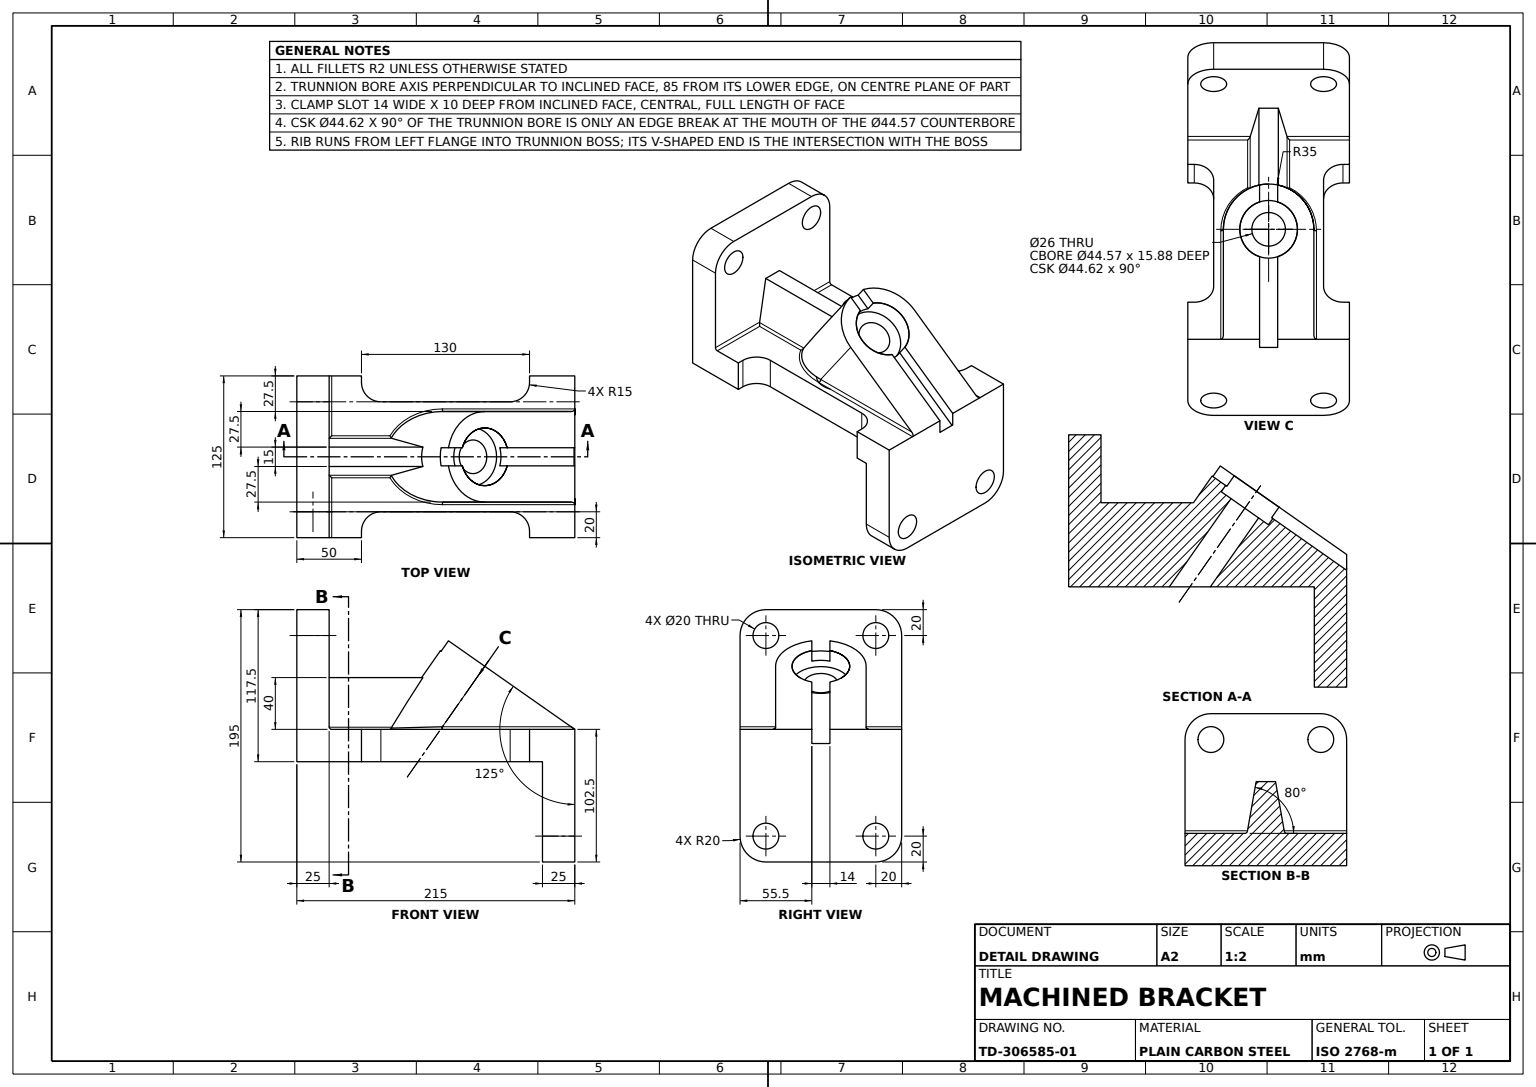
SolidWorks part; units mm, degrees
material "Plain Carbon Steel"
ref_plane "Front Plane" through (0, 0, 0) normal (0, 0, 1) x (1, 0, 0)
ref_plane "Top Plane" through (0, 0, 0) normal (0, 1, 0) x (1, 0, 0)
ref_plane "Right Plane" through (0, 0, 0) normal (1, 0, 0) x (0, 0, -1)
sketch "Base Plate Sketch" plane through (0, 0, 0) normal (0, 1, 0) x (1, 0, 0)
  line L0 (72.5, 62.5) -> (107.5, 62.5)
  line L1 (-107.5, -62.5) -> (-57.5, -62.5)
  line L2 (-107.5, -62.5) -> (-107.5, 62.5)
  line L3 (-107.5, 62.5) -> (-57.5, 62.5)
  line L4 (107.5, -62.5) -> (107.5, 62.5)
  line L5 (-107.5, -62.5) -> (107.5, 62.5) construction
  line L6 (-107.5, 62.5) -> (107.5, -62.5) construction
  line L8 (72.5, 62.5) -> (72.5, 57.5)
  line L9 (57.5, 42.5) -> (-42.5, 42.5)
  line L10 (-57.5, 62.5) -> (-57.5, 57.5)
  line L11 (0, 0) -> (-93.3615, 0) construction
  line L12 (-57.5, -62.5) -> (-57.5, -57.5)
  line L13 (72.5, -62.5) -> (72.5, -57.5)
  line L14 (57.5, -42.5) -> (-42.5, -42.5)
  line L15 (72.5, -62.5) -> (107.5, -62.5)
  arc A0 (-57.5, 57.5) -> (-42.5, 42.5) centre (-42.5, 57.5) ccw
  arc A1 (57.5, 42.5) -> (72.5, 57.5) centre (57.5, 57.5) ccw
  arc A2 (-57.5, -57.5) -> (-42.5, -42.5) centre (-42.5, -57.5) cw
  arc A3 (57.5, -42.5) -> (72.5, -57.5) centre (57.5, -57.5) cw
  point P0 (0, 0)
  point P13 (-57.5, 42.5)
  point P16 (72.5, 42.5)
  dimension "D5" = 15
  dimension "D1" = 215
  dimension "D2" = 125
  dimension "D3" = 20
  dimension "D4" = 100
  dimension "D6" = 50
extrude "Base Plate" add sketch "Base Plate Sketch" along normal blind 25
sketch "End Flange A Sketch" plane through (107.5, 0, 0) normal (1, 0, 0) x (0, 0, -1)
  line L0 (62.5, 25) -> (62.5, 0) construction
  line L1 (-62.5, 25) -> (62.5, 25)
  line L2 (-62.5, 25) -> (-62.5, -57.5)
  line L3 (-42.5, -77.5) -> (42.5, -77.5)
  line L4 (62.5, 25) -> (62.5, -57.5)
  arc A0 (62.5, -57.5) -> (42.5, -77.5) centre (42.5, -57.5) cw
  arc A1 (-42.5, -77.5) -> (-62.5, -57.5) centre (-42.5, -57.5) cw
  circle A2 centre (-42.5, -57.5) radius 10
  circle A3 centre (42.5, -57.5) radius 10
  dimension "D2" = 20
  dimension "D3" = 20
  dimension "D1" = 102.5
extrude "End Flange A" add sketch "End Flange A Sketch" against normal blind 25
sketch "End Flange B Sketch" plane through (-107.5, 0, 0) normal (-1, 0, 0) x (0, 0, 1)
  line L0 (62.5, 25) -> (62.5, 0) construction
  line L1 (-62.5, 0) -> (62.5, 0)
  line L2 (-62.5, 0) -> (-62.5, 97.5)
  line L3 (-42.5, 117.5) -> (42.5, 117.5)
  line L4 (62.5, 0) -> (62.5, 97.5)
  arc A0 (42.5, 117.5) -> (62.5, 97.5) centre (42.5, 97.5) cw
  arc A1 (-62.5, 97.5) -> (-42.5, 117.5) centre (-42.5, 97.5) cw
  circle A2 centre (-42.5, 97.5) radius 10
  circle A3 centre (42.5, 97.5) radius 10
  point P11 (-62.5, 117.5)
  dimension "D2" = 20
  dimension "D3" = 20
  dimension "D1" = 117.5
extrude "End Flange B" add sketch "End Flange B Sketch" against normal blind 25
ref_plane "Trunnion Plane 125deg" through (47.1126, 67.2837, 0) normal (-0.5736, -0.8192, 0) x (0, 0, -1)
sketch "Trunnion Boss Sketch" plane through (47.1126, 67.2837, 0) normal (-0.5736, -0.8192, 0) x (0, 0, -1)
  line L0 (-35, -11.2806) -> (-35, 73.7194)
  line L1 (-35, 73.7194) -> (35, 73.7194)
  line L2 (35, 73.7194) -> (35, -11.2806)
  line L5 (-62.5, 73.7194) -> (62.5, 73.7194) construction
  arc A0 (-35, -11.2806) -> (35, -11.2806) centre (0, -11.2806) ccw
  dimension "D1" = 70
  dimension "D2" = 85
extrude "Angled Trunnion Boss" add sketch "Trunnion Boss Sketch" along normal up to surface up to face at (8.75, 25, 0)
hole_wizard "Trunnion Bore CBORE M24" positions "3DSketch1" profile "Sketch6" counterbore size "M24" standard "ANSI Metric" end condition through all
sketch3d "3DSketch1"
  arc A0 (37.8721, 73.754, 35) -> (37.8721, 73.754, -35) centre (37.8721, 73.754, 0) ccw construction
  point P0 (37.8721, 73.754, 0)
  point P6 (17.7969, 45.0837, 0)
sketch "Sketch6" plane through (37.8721, 73.754, 0) normal (0, 0, 1) x (-0.8192, 0.5736, 0)
  line L0 (0, 0) -> (0, 207.282)
  line L1 (0, 207.282) -> (13, 207.282)
  line L3 (13, 207.282) -> (13, 15.9)
  line L4 (22.285, 15.9) -> (13, 15.9)
  line L5 (22.285, 15.9) -> (22.285, 0.025)
  line L6 (22.285, 0.025) -> (22.31, 0)
  line L7 (22.31, 0) -> (0, 0)
  line L8 (-22.285, 0.025) -> (-22.31, 0) construction
  line L11 (0, -6.35) -> (0, 107.95) construction
  dimension "Thru Hole Dia." = 26
  dimension "Thru Hole Depth" = 207.282
  dimension "C'Bore Dia." = 44.57
  dimension "C'Bore Depth" = 15.9
  dimension "Near C'Sink Dia." = 44.62
  dimension "Near C'Sink Angle" = 90
sketch "Clamp Slot Sketch" plane through (47.1126, 67.2837, 0) normal (0.5736, 0.8192, 0) x (0.8192, -0.5736, 0)
  line L1 (-55, 7) -> (80, 7)
  line L2 (-55, 7) -> (-55, -7)
  line L3 (-55, -7) -> (80, -7)
  line L4 (80, 7) -> (80, -7)
  point P5 (80, 0)
  dimension "D1" = 14
  dimension "D2" = 55
  dimension "D3" = 135
extrude "Clamp Slot 14mm" cut sketch "Clamp Slot Sketch" against normal blind 10
sketch "Support Rib Sketch" plane through (0, 0, 0) normal (0, 0, 1) x (1, 0, 0)
  line L0 (-82.5, 65) -> (-10.9846, 65)
  line L3 (-82.5, 25) -> (-82.5, 97.5) construction
  line L4 (3.466, 85.6377) -> (-38.993, 25) construction
  line L5 (-42.5, 25) -> (57.5, 25) construction
  dimension "D1" = 40
rib "Support Rib 15mm" sketch "Support Rib Sketch" sketch "Support Rib Sketch" thickness 15 extrusion direction parallel to sketch draft on yes draft angle 10 parameters "D1"=15, "D3"=10
fillet "Edge Fillets R2" radius 2 8 edges at (-19.3582, 25, 29.4479) (55.6171, 25, -35) (55.6171, 25, 35) (-58.8121, 25, 14.5531) (-82.5, 25, 38.5265) (-19.3582, 25, -29.4479) (-58.8121, 25, -14.5531) (-82.5, 25, -38.5265)
